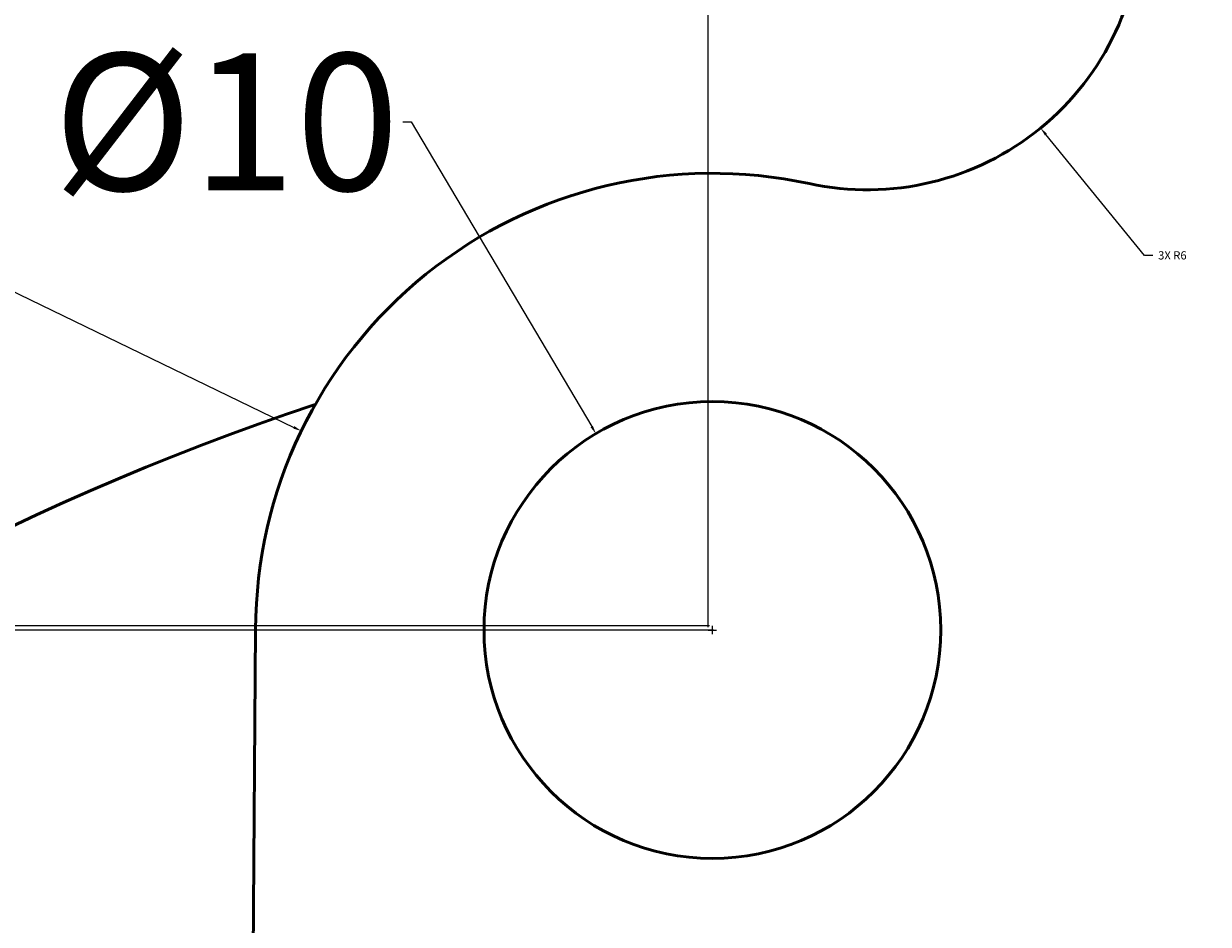
# Model space of a CAD drawing. Units: millimetres. Extents: x -53 to 92, y -147 to 37.
# Tile 12 of 16: x -6 to 20, y -10 to 9. Entities that reach past the tile are written whole.
import ezdxf

# ---------------------------------------------------------------- set-up
doc = ezdxf.new("R2010")
doc.units = ezdxf.units.MM
doc.header["$MEASUREMENT"] = 0
doc.layers.add('M-DIMS', color=2, linetype='Continuous', lineweight=25)
doc.layers.add('M-OUTL', color=7, linetype='Continuous', lineweight=50)
doc.styles.get("Standard").update_dxf_attribs({"font": 'arial.ttf'})
doc.dimstyles.get("Standard").update_dxf_attribs({"dimtxt": 0.18, "dimasz": 0.18, "dimexe": 0.18, "dimexo": 0.0625, "dimgap": 0.09, "dimtad": 0, "dimtih": 1, "dimtoh": 1, "dimdec": 4, "dimzin": 0, "dimdsep": 46, "dimtxsty": 'Standard', "dimcen": 0.09, "dimadec": 0, "dimazin": 0, "dimtfac": 1, "dimtdec": 4, "dimtofl": 0, "dimtmove": 0, "dimatfit": 3, "dimfxl": 1, "dimtolj": 1, "dimtzin": 0, "dimarcsym": 0})

# ---------------------------------------------------------------- blocks, each defined once
blk = doc.blocks.new('*D2')
at = {"layer": 'Defpoints', "color": 0, "transparency": 16777216}
for p in [(0.354, 0.478), (9.355, -3.88)]:
    blk.add_point(p, dxfattribs=at)
at = {"layer": 'M-DIMS', "color": 0, "lineweight": -2, "transparency": 16777216}
for p, q in [((-13.114, 6.912), (-12.934, 6.912)), ((-12.934, 6.912), (0.192, 0.557)), ((9.265, -3.88), (9.445, -3.88)), ((9.355, -3.97), (9.355, -3.79))]:
    blk.add_line(p, q, dxfattribs=at)
at = {"layer": 'M-DIMS', "color": 0, "transparency": 16777216}
blk.add_solid([(0.205, 0.584), (0.179, 0.53), (0.354, 0.478)], dxfattribs=at)
at = {"layer": 'M-DIMS', "color": 0, "transparency": 16777216, "insert": (-16.783, 6.912), "char_height": 0.18, "attachment_point": 5}
blk.add_mtext('\\A1;{\\H16.66667x;R10}', dxfattribs=at)
blk = doc.blocks.new('*D4')
at = {"layer": 'Defpoints', "color": 0, "transparency": 16777216}
for p in [(6.804, 0.421), (11.905, -8.18)]:
    blk.add_point(p, dxfattribs=at)
at = {"layer": 'M-DIMS', "color": 0, "lineweight": -2, "transparency": 16777216}
for p, q in [((2.577, 7.244), (2.757, 7.244)), ((2.757, 7.244), (6.712, 0.576)), ((9.265, -3.88), (9.445, -3.88)), ((9.355, -3.97), (9.355, -3.79))]:
    blk.add_line(p, q, dxfattribs=at)
at = {"layer": 'M-DIMS', "color": 0, "transparency": 16777216}
blk.add_solid([(6.738, 0.591), (6.686, 0.56), (6.804, 0.421)], dxfattribs=at)
at = {"layer": 'M-DIMS', "color": 0, "transparency": 16777216, "insert": (-1.289, 7.244), "char_height": 0.18, "attachment_point": 5}
blk.add_mtext('\\A1;{\\H16.66667x;%%C10}', dxfattribs=at)
blk = doc.blocks.new('*D5')
at = {"layer": 'Defpoints', "color": 0, "transparency": 16777216}
for p in [(28.602, 35.845), (28.602, 15.91), (9.265, -3.88)]:
    blk.add_point(p, dxfattribs=at)
at = {"layer": 'M-DIMS', "color": 0, "lineweight": -2, "transparency": 16777216}
for p, q in [((9.265, -3.817), (9.265, 36.025)), ((9.445, 35.845), (16.674, 35.845)), ((28.422, 35.845), (21.192, 35.845)), ((28.602, 15.973), (28.602, 36.025))]:
    blk.add_line(p, q, dxfattribs=at)
at = {"layer": 'M-DIMS', "color": 0, "transparency": 16777216}
for points in [[(9.445, 35.875), (9.445, 35.815), (9.265, 35.845)], [(28.422, 35.875), (28.422, 35.815), (28.602, 35.845)]]:
    blk.add_solid(points, dxfattribs=at)
at = {"layer": 'M-DIMS', "color": 0, "transparency": 16777216, "insert": (18.933, 35.845), "char_height": 0.18, "attachment_point": 5}
blk.add_mtext('\\A1;{\\H16.66667x;20}', dxfattribs=at)
blk = doc.blocks.new('*D6')
at = {"layer": 'Defpoints', "color": 0, "transparency": 16777216}
for p in [(-26.95, 15.91), (28.602, 15.91), (9.355, -3.79)]:
    blk.add_point(p, dxfattribs=at)
at = {"layer": 'M-DIMS', "color": 0, "lineweight": -2, "transparency": 16777216}
for p, q in [((28.539, 15.91), (-27.13, 15.91)), ((-26.95, 15.73), (-26.95, 7.682)), ((-26.95, -3.61), (-26.95, 4.438)), ((9.292, -3.79), (-27.13, -3.79))]:
    blk.add_line(p, q, dxfattribs=at)
at = {"layer": 'M-DIMS', "color": 0, "transparency": 16777216}
for points in [[(-26.98, 15.73), (-26.92, 15.73), (-26.95, 15.91)], [(-26.98, -3.61), (-26.92, -3.61), (-26.95, -3.79)]]:
    blk.add_solid(points, dxfattribs=at)
at = {"layer": 'M-DIMS', "color": 0, "transparency": 16777216, "insert": (-26.95, 6.06), "char_height": 0.18, "attachment_point": 5}
blk.add_mtext('\\A1;{\\H16.66667x;20}', dxfattribs=at)
blk = doc.blocks.new('*D7')
at = {"layer": 'Defpoints', "color": 0, "transparency": 16777216}
for p in [(9.445, -3.88), (-44.321, -53.98), (18.956, -53.98)]:
    blk.add_point(p, dxfattribs=at)
at = {"layer": 'M-DIMS', "color": 0, "lineweight": -2, "transparency": 16777216}
for p, q in [((9.382, -3.88), (-44.501, -3.88)), ((-44.321, -4.06), (-44.321, -27.308)), ((-44.321, -53.8), (-44.321, -30.552)), ((18.894, -53.98), (-44.501, -53.98))]:
    blk.add_line(p, q, dxfattribs=at)
at = {"layer": 'M-DIMS', "color": 0, "transparency": 16777216}
for points in [[(-44.351, -4.06), (-44.291, -4.06), (-44.321, -3.88)], [(-44.351, -53.8), (-44.291, -53.8), (-44.321, -53.98)]]:
    blk.add_solid(points, dxfattribs=at)
at = {"layer": 'M-DIMS', "color": 0, "transparency": 16777216, "insert": (-44.321, -28.93), "char_height": 0.18, "attachment_point": 5}
blk.add_mtext('\\A1;{\\H16.66667x;50}', dxfattribs=at)
blk = doc.blocks.new('*D10')
at = {"layer": 'Defpoints', "color": 0, "transparency": 16777216}
for p in [(64.593, -18.184), (-26.68, -89.776)]:
    blk.add_point(p, dxfattribs=at)
at = {"layer": 'M-DIMS', "color": 0, "lineweight": -2, "transparency": 16777216}
for p, q in [((77.384, -8.151), (64.734, -18.073)), ((77.564, -8.151), (77.384, -8.151)), ((18.956, -54.07), (18.956, -53.89)), ((18.866, -53.98), (19.046, -53.98))]:
    blk.add_line(p, q, dxfattribs=at)
at = {"layer": 'M-DIMS', "color": 0, "transparency": 16777216}
blk.add_solid([(64.716, -18.05), (64.753, -18.097), (64.593, -18.184)], dxfattribs=at)
at = {"layer": 'M-DIMS', "color": 0, "transparency": 16777216, "insert": (82.599, -8.151), "char_height": 0.18, "attachment_point": 5}
blk.add_mtext('\\A1;{\\H16.66667x;%%C116}', dxfattribs=at)
blk = doc.blocks.new('HOLE-D10')
blk.add_circle((5, 5), 5)
blk = doc.blocks.new('*D17')
at = {"layer": 'Defpoints', "color": 0, "transparency": 16777216}
for p in [(-46.81, 25.909), (28.564, 25.909), (18.165, -111.975)]:
    blk.add_point(p, dxfattribs=at)
at = {"layer": 'M-DIMS', "color": 0, "lineweight": -2, "transparency": 16777216}
for p, q in [((28.502, 25.909), (-46.99, 25.909)), ((-46.81, 25.729), (-46.81, -42.851)), ((-46.81, -111.795), (-46.81, -43.215)), ((18.102, -111.975), (-46.99, -111.975))]:
    blk.add_line(p, q, dxfattribs=at)
at = {"layer": 'M-DIMS', "color": 0, "transparency": 16777216}
for points in [[(-46.84, 25.729), (-46.78, 25.729), (-46.81, 25.909)], [(-46.84, -111.795), (-46.78, -111.795), (-46.81, -111.975)]]:
    blk.add_solid(points, dxfattribs=at)
at = {"layer": 'M-DIMS', "color": 0, "transparency": 16777216, "insert": (-46.81, -43.033), "char_height": 0.18, "attachment_point": 5}
blk.add_mtext('\\A1;137.88', dxfattribs=at)
blk = doc.blocks.new('*D18')
at = {"layer": 'Defpoints', "color": 0, "transparency": 16777216}
for p in [(19.753, 4.014), (18.16, -111.975)]:
    blk.add_point(p, dxfattribs=at)
at = {"layer": 'M-DIMS', "color": 0, "lineweight": -2, "transparency": 16777216}
for p, q in [((18.956, -54.07), (18.956, -53.89)), ((18.866, -53.98), (19.046, -53.98)), ((17.682, -146.771), (18.158, -112.155)), ((17.502, -146.771), (17.682, -146.771))]:
    blk.add_line(p, q, dxfattribs=at)
at = {"layer": 'M-DIMS', "color": 0, "transparency": 16777216}
blk.add_solid([(18.128, -112.154), (18.188, -112.155), (18.16, -111.975)], dxfattribs=at)
at = {"layer": 'M-DIMS', "color": 0, "transparency": 16777216, "insert": (17.115, -146.771), "char_height": 0.18, "attachment_point": 5}
blk.add_mtext('\\A1;∅116', dxfattribs=at)
blk = doc.blocks.new('*D21')
at = {"layer": 'Defpoints', "color": 0, "transparency": 16777216}
for p in [(12.745, 11.757), (16.541, 7.111)]:
    blk.add_point(p, dxfattribs=at)
at = {"layer": 'M-DIMS', "color": 0, "lineweight": -2, "transparency": 16777216}
for p, q in [((12.655, 11.757), (12.835, 11.757)), ((12.745, 11.667), (12.745, 11.847)), ((18.819, 4.323), (16.655, 6.971)), ((18.999, 4.323), (18.819, 4.323))]:
    blk.add_line(p, q, dxfattribs=at)
at = {"layer": 'M-DIMS', "color": 0, "transparency": 16777216}
blk.add_solid([(16.678, 6.99), (16.632, 6.953), (16.541, 7.111)], dxfattribs=at)
at = {"layer": 'M-DIMS', "color": 0, "transparency": 16777216, "insert": (19.427, 4.323), "char_height": 0.18, "attachment_point": 5}
blk.add_mtext('\\A1;3X R6', dxfattribs=at)

msp = doc.modelspace()

# ---------------------------------------------------------------- linework, layer by layer
at = {"layer": 'M-OUTL'}
msp.add_line((-1.07952, -58.41764), (-0.64538, -3.86515), dxfattribs=at)
for centre, radius, start, end in [((12.74458, 11.75699), 6, 257.767876, 0.732363), ((9.35461, -3.87977), 10, 77.767876, 179.916244), ((18.95638, -53.98007), 58, 108.3895553, 70.0459142)]:
    msp.add_arc(centre, radius, start, end, dxfattribs=at)

# ---------------------------------------------------------------- block references
msp.add_blockref('HOLE-D10', (4.35473, -8.87982), dxfattribs=at)

# ---------------------------------------------------------------- dimensions: what is measured, and where the dimension line sits
at = {"layer": 'M-DIMS'}
dim = msp.add_linear_dim(base=(28.60189, 35.84496), p1=(9.26461, -3.87977), p2=(28.60189, 15.91006), text='{\\H16.66667x;20}', dimstyle='Standard', override={"dimclrd": 0, "dimclre": 0, "dimclrt": 0}, dxfattribs=at)
dim.commit()
dim.dimension.update_dxf_attribs({"geometry": '*D5', "text_midpoint": (18.93325, 35.84496)})
dim = msp.add_linear_dim(base=(-46.8103, 25.90924), p1=(18.16452, -111.97467), p2=(28.56407, 25.90924), angle=90, dimstyle='Standard', override={"dimdec": 2, "dimlfac": 1, "dimrnd": 0, "dimzin": 0, "dimdsep": 46, "dimlunit": 2}, dxfattribs=at)
dim.commit()
dim.dimension.update_dxf_attribs({"geometry": '*D17', "text_midpoint": (-46.8103, -43.03271)})
for base, p1, p2, text, picture, middle in [((-26.95014, 15.91006), (9.35461, -3.78977), (28.60189, 15.91006), '{\\H16.66667x;20}', '*D6', (-26.95014, 6.06014)), ((-44.32095, -53.98007), (9.44461, -3.87977), (18.95638, -53.98007), '{\\H16.66667x;50}', '*D7', (-44.32095, -28.92992))]:
    dim = msp.add_linear_dim(base=base, p1=p1, p2=p2, angle=90, text=text, dimstyle='Standard', override={"dimclrd": 0, "dimclre": 0, "dimclrt": 0}, dxfattribs=at)
    dim.commit()
    dim.dimension.update_dxf_attribs({"geometry": picture, "text_midpoint": middle})
for center, mpoint, text, override, picture, middle in [((12.74458, 11.75699), (16.5411, 7.11087), '3X <>', {"dimdec": 0, "dimlfac": 1, "dimrnd": 0, "dimzin": 0, "dimdsep": 46, "dimlunit": 2}, '*D21', (19.42741, 4.3232)), ((9.35461, -3.87977), (0.35416, 0.47819), '{\\H16.66667x;R10}', {"dimclrd": 0, "dimclre": 0, "dimclrt": 0}, '*D2', (-16.78265, 6.912))]:
    dim = msp.add_radius_dim(center=center, mpoint=mpoint, text=text, dimstyle='Standard', override=override, dxfattribs=at)
    dim.commit()
    dim.dimension.update_dxf_attribs({"geometry": picture, "text_midpoint": middle, "dimtype": 164})
for p1, p2, text, picture, middle in [((11.90526, -8.18026), (6.80397, 0.42072), '{\\H16.66667x;%%C10}', '*D4', (-1.28855, 7.24403)), ((-26.67986, -89.77579), (64.59262, -18.18435), '{\\H16.66667x;%%C116}', '*D10', (82.59889, -8.15132))]:
    dim = msp.add_diameter_dim_2p(p1=p1, p2=p2, text=text, dimstyle='Standard', override={"dimclrd": 0, "dimclre": 0, "dimclrt": 0}, dxfattribs=at)
    dim.commit()
    dim.dimension.update_dxf_attribs({"geometry": picture, "text_midpoint": middle, "dimtype": 163})
dim = msp.add_diameter_dim_2p(p1=(19.75275, 4.01446), p2=(18.16001, -111.9746), dimstyle='Standard', override={"dimdec": 0, "dimlfac": 1, "dimrnd": 0, "dimzin": 0, "dimdsep": 46, "dimlunit": 2}, dxfattribs=at)
dim.commit()
dim.dimension.update_dxf_attribs({"geometry": '*D18', "text_midpoint": (17.11548, -146.77132), "dimtype": 163})

doc.saveas('drawing.dxf')
